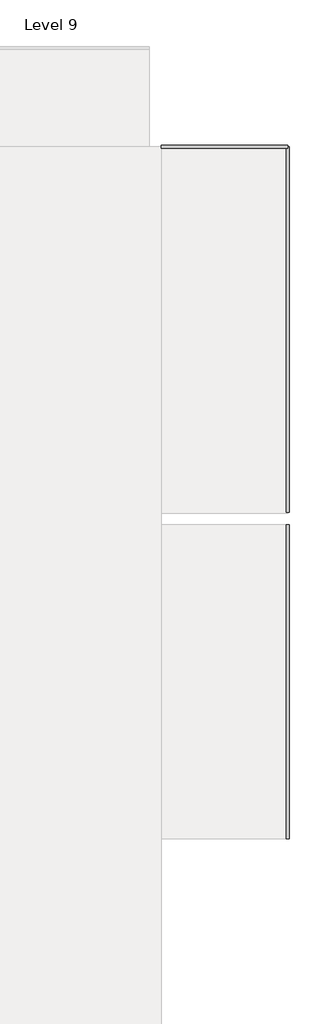
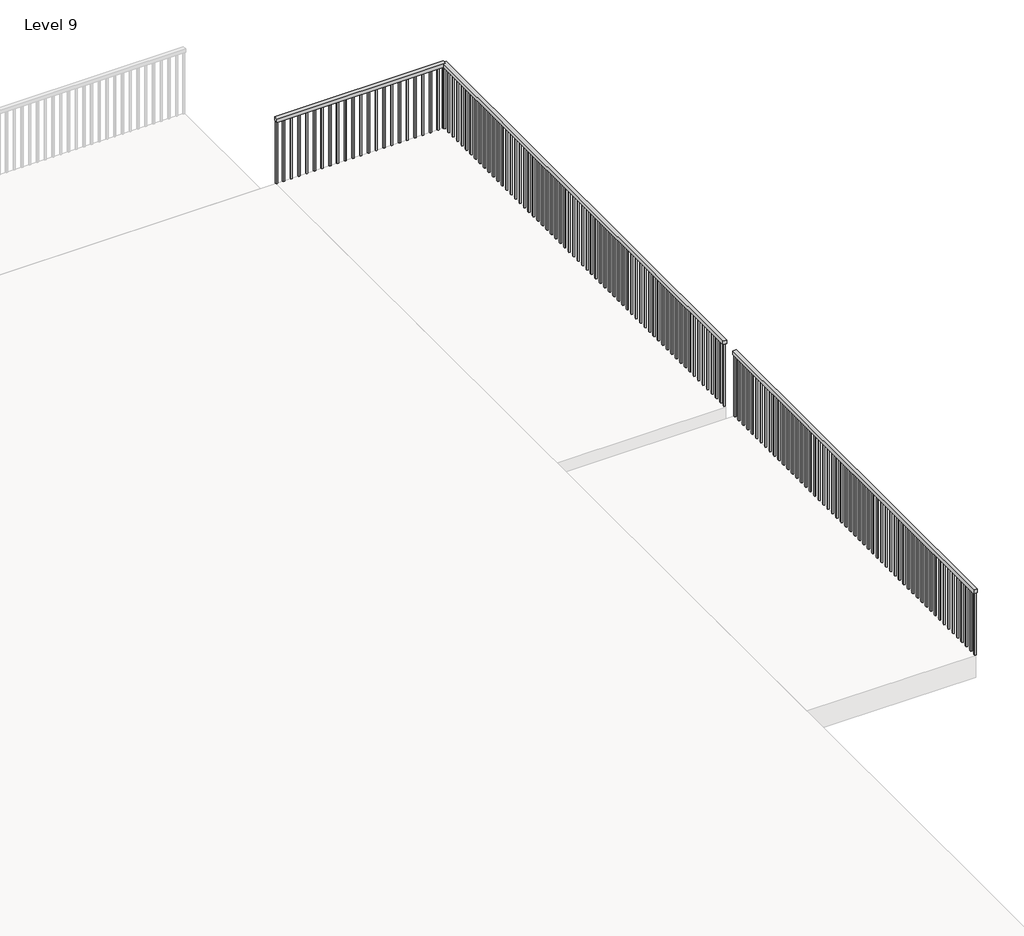
# One storey, part 4 of 5: 3 railings.
"""IFC4 building model written with IfcOpenShell, lengths in millimetres."""

from ifc_helpers import new_model, si_unit, frame, origin, place, context, project, spatial, polyline, outline, extrude, element, save

model = new_model("IFC4")

# Units and contexts
model_context = context("Model", 3, world=origin())
ifc_project = project(units=[si_unit("LENGTHUNIT", "METRE", prefix="MILLI")], contexts=[model_context])

# Site, building, storey
site = spatial("IfcSite", under=ifc_project)
building = spatial("IfcBuilding", under=site)
storey = spatial("IfcBuildingStorey", under=building, Name="Level 9", Elevation=9448.8)

# Railings
placement = place(None, origin())
element("IfcRailing", 1, ObjectType="Handrail - Rectangular", at=placement, inside=storey, context=model_context, shape_type="SweptSolid", body=[
    extrude(outline(polyline([(14106.5361222, 14743.2237525), (14106.5361222, 14794.0237525), (16321.4289933, 14794.0237525), (16321.4289933, 14743.2237525), (14106.5361222, 14743.2237525)])), frame((0.0, 0.0, 10312.4), z_axis=(0.0, 0.0, 1.0), x_axis=(1.0, 0.0, 0.0)), (0.0, 0.0, 1.0), 50.8),
    extrude(outline(polyline([(16230.6111222, 14759.0987525), (16230.6111222, 14778.1487525), (16249.6611222, 14778.1487525), (16249.6611222, 14759.0987525), (16230.6111222, 14759.0987525)])), frame((0.0, 0.0, 9448.8), z_axis=(0.0, 0.0, 1.0), x_axis=(1.0, 0.0, 0.0)), (0.0, 0.0, 1.0), 863.6),
    extrude(outline(polyline([(16129.0111222, 14759.0987525), (16129.0111222, 14778.1487525), (16148.0611222, 14778.1487525), (16148.0611222, 14759.0987525), (16129.0111222, 14759.0987525)])), frame((0.0, 0.0, 9448.8), z_axis=(0.0, 0.0, 1.0), x_axis=(1.0, 0.0, 0.0)), (0.0, 0.0, 1.0), 863.6),
    extrude(outline(polyline([(16027.4111222, 14759.0987525), (16027.4111222, 14778.1487525), (16046.4611222, 14778.1487525), (16046.4611222, 14759.0987525), (16027.4111222, 14759.0987525)])), frame((0.0, 0.0, 9448.8), z_axis=(0.0, 0.0, 1.0), x_axis=(1.0, 0.0, 0.0)), (0.0, 0.0, 1.0), 863.6),
    extrude(outline(polyline([(15925.8111222, 14759.0987525), (15925.8111222, 14778.1487525), (15944.8611222, 14778.1487525), (15944.8611222, 14759.0987525), (15925.8111222, 14759.0987525)])), frame((0.0, 0.0, 9448.8), z_axis=(0.0, 0.0, 1.0), x_axis=(1.0, 0.0, 0.0)), (0.0, 0.0, 1.0), 863.6),
    extrude(outline(polyline([(15824.2111222, 14759.0987525), (15824.2111222, 14778.1487525), (15843.2611222, 14778.1487525), (15843.2611222, 14759.0987525), (15824.2111222, 14759.0987525)])), frame((0.0, 0.0, 9448.8), z_axis=(0.0, 0.0, 1.0), x_axis=(1.0, 0.0, 0.0)), (0.0, 0.0, 1.0), 863.6),
    extrude(outline(polyline([(15722.6111222, 14759.0987525), (15722.6111222, 14778.1487525), (15741.6611222, 14778.1487525), (15741.6611222, 14759.0987525), (15722.6111222, 14759.0987525)])), frame((0.0, 0.0, 9448.8), z_axis=(0.0, 0.0, 1.0), x_axis=(1.0, 0.0, 0.0)), (0.0, 0.0, 1.0), 863.6),
    extrude(outline(polyline([(15621.0111222, 14759.0987525), (15621.0111222, 14778.1487525), (15640.0611222, 14778.1487525), (15640.0611222, 14759.0987525), (15621.0111222, 14759.0987525)])), frame((0.0, 0.0, 9448.8), z_axis=(0.0, 0.0, 1.0), x_axis=(1.0, 0.0, 0.0)), (0.0, 0.0, 1.0), 863.6),
    extrude(outline(polyline([(15519.4111222, 14759.0987525), (15519.4111222, 14778.1487525), (15538.4611222, 14778.1487525), (15538.4611222, 14759.0987525), (15519.4111222, 14759.0987525)])), frame((0.0, 0.0, 9448.8), z_axis=(0.0, 0.0, 1.0), x_axis=(1.0, 0.0, 0.0)), (0.0, 0.0, 1.0), 863.6),
    extrude(outline(polyline([(15417.8111222, 14759.0987525), (15417.8111222, 14778.1487525), (15436.8611222, 14778.1487525), (15436.8611222, 14759.0987525), (15417.8111222, 14759.0987525)])), frame((0.0, 0.0, 9448.8), z_axis=(0.0, 0.0, 1.0), x_axis=(1.0, 0.0, 0.0)), (0.0, 0.0, 1.0), 863.6),
    extrude(outline(polyline([(15316.2111222, 14759.0987525), (15316.2111222, 14778.1487525), (15335.2611222, 14778.1487525), (15335.2611222, 14759.0987525), (15316.2111222, 14759.0987525)])), frame((0.0, 0.0, 9448.8), z_axis=(0.0, 0.0, 1.0), x_axis=(1.0, 0.0, 0.0)), (0.0, 0.0, 1.0), 863.6),
    extrude(outline(polyline([(15214.6111222, 14759.0987525), (15214.6111222, 14778.1487525), (15233.6611222, 14778.1487525), (15233.6611222, 14759.0987525), (15214.6111222, 14759.0987525)])), frame((0.0, 0.0, 9448.8), z_axis=(0.0, 0.0, 1.0), x_axis=(1.0, 0.0, 0.0)), (0.0, 0.0, 1.0), 863.6),
    extrude(outline(polyline([(15113.0111222, 14759.0987525), (15113.0111222, 14778.1487525), (15132.0611222, 14778.1487525), (15132.0611222, 14759.0987525), (15113.0111222, 14759.0987525)])), frame((0.0, 0.0, 9448.8), z_axis=(0.0, 0.0, 1.0), x_axis=(1.0, 0.0, 0.0)), (0.0, 0.0, 1.0), 863.6),
    extrude(outline(polyline([(15011.4111222, 14759.0987525), (15011.4111222, 14778.1487525), (15030.4611222, 14778.1487525), (15030.4611222, 14759.0987525), (15011.4111222, 14759.0987525)])), frame((0.0, 0.0, 9448.8), z_axis=(0.0, 0.0, 1.0), x_axis=(1.0, 0.0, 0.0)), (0.0, 0.0, 1.0), 863.6),
    extrude(outline(polyline([(14909.8111222, 14759.0987525), (14909.8111222, 14778.1487525), (14928.8611222, 14778.1487525), (14928.8611222, 14759.0987525), (14909.8111222, 14759.0987525)])), frame((0.0, 0.0, 9448.8), z_axis=(0.0, 0.0, 1.0), x_axis=(1.0, 0.0, 0.0)), (0.0, 0.0, 1.0), 863.6),
    extrude(outline(polyline([(14808.2111222, 14759.0987525), (14808.2111222, 14778.1487525), (14827.2611222, 14778.1487525), (14827.2611222, 14759.0987525), (14808.2111222, 14759.0987525)])), frame((0.0, 0.0, 9448.8), z_axis=(0.0, 0.0, 1.0), x_axis=(1.0, 0.0, 0.0)), (0.0, 0.0, 1.0), 863.6),
    extrude(outline(polyline([(14706.6111222, 14759.0987525), (14706.6111222, 14778.1487525), (14725.6611222, 14778.1487525), (14725.6611222, 14759.0987525), (14706.6111222, 14759.0987525)])), frame((0.0, 0.0, 9448.8), z_axis=(0.0, 0.0, 1.0), x_axis=(1.0, 0.0, 0.0)), (0.0, 0.0, 1.0), 863.6),
    extrude(outline(polyline([(14605.0111222, 14759.0987525), (14605.0111222, 14778.1487525), (14624.0611222, 14778.1487525), (14624.0611222, 14759.0987525), (14605.0111222, 14759.0987525)])), frame((0.0, 0.0, 9448.8), z_axis=(0.0, 0.0, 1.0), x_axis=(1.0, 0.0, 0.0)), (0.0, 0.0, 1.0), 863.6),
    extrude(outline(polyline([(14503.4111222, 14759.0987525), (14503.4111222, 14778.1487525), (14522.4611222, 14778.1487525), (14522.4611222, 14759.0987525), (14503.4111222, 14759.0987525)])), frame((0.0, 0.0, 9448.8), z_axis=(0.0, 0.0, 1.0), x_axis=(1.0, 0.0, 0.0)), (0.0, 0.0, 1.0), 863.6),
    extrude(outline(polyline([(14401.8111222, 14759.0987525), (14401.8111222, 14778.1487525), (14420.8611222, 14778.1487525), (14420.8611222, 14759.0987525), (14401.8111222, 14759.0987525)])), frame((0.0, 0.0, 9448.8), z_axis=(0.0, 0.0, 1.0), x_axis=(1.0, 0.0, 0.0)), (0.0, 0.0, 1.0), 863.6),
    extrude(outline(polyline([(14300.2111222, 14759.0987525), (14300.2111222, 14778.1487525), (14319.2611222, 14778.1487525), (14319.2611222, 14759.0987525), (14300.2111222, 14759.0987525)])), frame((0.0, 0.0, 9448.8), z_axis=(0.0, 0.0, 1.0), x_axis=(1.0, 0.0, 0.0)), (0.0, 0.0, 1.0), 863.6),
    extrude(outline(polyline([(14198.6111222, 14759.0987525), (14198.6111222, 14778.1487525), (14217.6611222, 14778.1487525), (14217.6611222, 14759.0987525), (14198.6111222, 14759.0987525)])), frame((0.0, 0.0, 9448.8), z_axis=(0.0, 0.0, 1.0), x_axis=(1.0, 0.0, 0.0)), (0.0, 0.0, 1.0), 863.6),
    extrude(outline(polyline([(16302.3789933, 14759.0987525), (16302.3789933, 14778.1487525), (16321.4289933, 14778.1487525), (16321.4289933, 14759.0987525), (16302.3789933, 14759.0987525)])), frame((0.0, 0.0, 9448.8), z_axis=(0.0, 0.0, 1.0), x_axis=(1.0, 0.0, 0.0)), (0.0, 0.0, 1.0), 863.6),
    extrude(outline(polyline([(14106.5361222, 14759.0987525), (14106.5361222, 14778.1487525), (14125.5861222, 14778.1487525), (14125.5861222, 14759.0987525), (14106.5361222, 14759.0987525)])), frame((0.0, 0.0, 9448.8), z_axis=(0.0, 0.0, 1.0), x_axis=(1.0, 0.0, 0.0)), (0.0, 0.0, 1.0), 863.6),
])
element("IfcRailing", 2, ObjectType="Handrail - Rectangular", at=placement, inside=storey, context=model_context, shape_type="SweptSolid", body=[
    extrude(outline(polyline([(16296.0289933, 14768.6237525), (16346.8289933, 14768.6237525), (16346.8289933, 8386.8737525), (16296.0289933, 8386.8737525), (16296.0289933, 14768.6237525)])), frame((0.0, 0.0, 10312.4), z_axis=(0.0, 0.0, 1.0), x_axis=(1.0, 0.0, 0.0)), (0.0, 0.0, 1.0), 50.8),
    extrude(outline(polyline([(16311.9039933, 8478.9487525), (16330.9539933, 8478.9487525), (16330.9539933, 8459.8987525), (16311.9039933, 8459.8987525), (16311.9039933, 8478.9487525)])), frame((0.0, 0.0, 9448.8), z_axis=(0.0, 0.0, 1.0), x_axis=(1.0, 0.0, 0.0)), (0.0, 0.0, 1.0), 863.6),
    extrude(outline(polyline([(16311.9039933, 8580.5487525), (16330.9539933, 8580.5487525), (16330.9539933, 8561.4987525), (16311.9039933, 8561.4987525), (16311.9039933, 8580.5487525)])), frame((0.0, 0.0, 9448.8), z_axis=(0.0, 0.0, 1.0), x_axis=(1.0, 0.0, 0.0)), (0.0, 0.0, 1.0), 863.6),
    extrude(outline(polyline([(16311.9039933, 8682.1487525), (16330.9539933, 8682.1487525), (16330.9539933, 8663.0987525), (16311.9039933, 8663.0987525), (16311.9039933, 8682.1487525)])), frame((0.0, 0.0, 9448.8), z_axis=(0.0, 0.0, 1.0), x_axis=(1.0, 0.0, 0.0)), (0.0, 0.0, 1.0), 863.6),
    extrude(outline(polyline([(16311.9039933, 8783.7487525), (16330.9539933, 8783.7487525), (16330.9539933, 8764.6987525), (16311.9039933, 8764.6987525), (16311.9039933, 8783.7487525)])), frame((0.0, 0.0, 9448.8), z_axis=(0.0, 0.0, 1.0), x_axis=(1.0, 0.0, 0.0)), (0.0, 0.0, 1.0), 863.6),
    extrude(outline(polyline([(16311.9039933, 8885.3487525), (16330.9539933, 8885.3487525), (16330.9539933, 8866.2987525), (16311.9039933, 8866.2987525), (16311.9039933, 8885.3487525)])), frame((0.0, 0.0, 9448.8), z_axis=(0.0, 0.0, 1.0), x_axis=(1.0, 0.0, 0.0)), (0.0, 0.0, 1.0), 863.6),
    extrude(outline(polyline([(16311.9039933, 8986.9487525), (16330.9539933, 8986.9487525), (16330.9539933, 8967.8987525), (16311.9039933, 8967.8987525), (16311.9039933, 8986.9487525)])), frame((0.0, 0.0, 9448.8), z_axis=(0.0, 0.0, 1.0), x_axis=(1.0, 0.0, 0.0)), (0.0, 0.0, 1.0), 863.6),
    extrude(outline(polyline([(16311.9039933, 9088.5487525), (16330.9539933, 9088.5487525), (16330.9539933, 9069.4987525), (16311.9039933, 9069.4987525), (16311.9039933, 9088.5487525)])), frame((0.0, 0.0, 9448.8), z_axis=(0.0, 0.0, 1.0), x_axis=(1.0, 0.0, 0.0)), (0.0, 0.0, 1.0), 863.6),
    extrude(outline(polyline([(16311.9039933, 9190.1487525), (16330.9539933, 9190.1487525), (16330.9539933, 9171.0987525), (16311.9039933, 9171.0987525), (16311.9039933, 9190.1487525)])), frame((0.0, 0.0, 9448.8), z_axis=(0.0, 0.0, 1.0), x_axis=(1.0, 0.0, 0.0)), (0.0, 0.0, 1.0), 863.6),
    extrude(outline(polyline([(16311.9039933, 9291.7487525), (16330.9539933, 9291.7487525), (16330.9539933, 9272.6987525), (16311.9039933, 9272.6987525), (16311.9039933, 9291.7487525)])), frame((0.0, 0.0, 9448.8), z_axis=(0.0, 0.0, 1.0), x_axis=(1.0, 0.0, 0.0)), (0.0, 0.0, 1.0), 863.6),
    extrude(outline(polyline([(16311.9039933, 9393.3487525), (16330.9539933, 9393.3487525), (16330.9539933, 9374.2987525), (16311.9039933, 9374.2987525), (16311.9039933, 9393.3487525)])), frame((0.0, 0.0, 9448.8), z_axis=(0.0, 0.0, 1.0), x_axis=(1.0, 0.0, 0.0)), (0.0, 0.0, 1.0), 863.6),
    extrude(outline(polyline([(16311.9039933, 9494.9487525), (16330.9539933, 9494.9487525), (16330.9539933, 9475.8987525), (16311.9039933, 9475.8987525), (16311.9039933, 9494.9487525)])), frame((0.0, 0.0, 9448.8), z_axis=(0.0, 0.0, 1.0), x_axis=(1.0, 0.0, 0.0)), (0.0, 0.0, 1.0), 863.6),
    extrude(outline(polyline([(16311.9039933, 9596.5487525), (16330.9539933, 9596.5487525), (16330.9539933, 9577.4987525), (16311.9039933, 9577.4987525), (16311.9039933, 9596.5487525)])), frame((0.0, 0.0, 9448.8), z_axis=(0.0, 0.0, 1.0), x_axis=(1.0, 0.0, 0.0)), (0.0, 0.0, 1.0), 863.6),
    extrude(outline(polyline([(16311.9039933, 9698.1487525), (16330.9539933, 9698.1487525), (16330.9539933, 9679.0987525), (16311.9039933, 9679.0987525), (16311.9039933, 9698.1487525)])), frame((0.0, 0.0, 9448.8), z_axis=(0.0, 0.0, 1.0), x_axis=(1.0, 0.0, 0.0)), (0.0, 0.0, 1.0), 863.6),
    extrude(outline(polyline([(16311.9039933, 9799.7487525), (16330.9539933, 9799.7487525), (16330.9539933, 9780.6987525), (16311.9039933, 9780.6987525), (16311.9039933, 9799.7487525)])), frame((0.0, 0.0, 9448.8), z_axis=(0.0, 0.0, 1.0), x_axis=(1.0, 0.0, 0.0)), (0.0, 0.0, 1.0), 863.6),
    extrude(outline(polyline([(16311.9039933, 9901.3487525), (16330.9539933, 9901.3487525), (16330.9539933, 9882.2987525), (16311.9039933, 9882.2987525), (16311.9039933, 9901.3487525)])), frame((0.0, 0.0, 9448.8), z_axis=(0.0, 0.0, 1.0), x_axis=(1.0, 0.0, 0.0)), (0.0, 0.0, 1.0), 863.6),
    extrude(outline(polyline([(16311.9039933, 10002.9487525), (16330.9539933, 10002.9487525), (16330.9539933, 9983.8987525), (16311.9039933, 9983.8987525), (16311.9039933, 10002.9487525)])), frame((0.0, 0.0, 9448.8), z_axis=(0.0, 0.0, 1.0), x_axis=(1.0, 0.0, 0.0)), (0.0, 0.0, 1.0), 863.6),
    extrude(outline(polyline([(16311.9039933, 10104.5487525), (16330.9539933, 10104.5487525), (16330.9539933, 10085.4987525), (16311.9039933, 10085.4987525), (16311.9039933, 10104.5487525)])), frame((0.0, 0.0, 9448.8), z_axis=(0.0, 0.0, 1.0), x_axis=(1.0, 0.0, 0.0)), (0.0, 0.0, 1.0), 863.6),
    extrude(outline(polyline([(16311.9039933, 10206.1487525), (16330.9539933, 10206.1487525), (16330.9539933, 10187.0987525), (16311.9039933, 10187.0987525), (16311.9039933, 10206.1487525)])), frame((0.0, 0.0, 9448.8), z_axis=(0.0, 0.0, 1.0), x_axis=(1.0, 0.0, 0.0)), (0.0, 0.0, 1.0), 863.6),
    extrude(outline(polyline([(16311.9039933, 10307.7487525), (16330.9539933, 10307.7487525), (16330.9539933, 10288.6987525), (16311.9039933, 10288.6987525), (16311.9039933, 10307.7487525)])), frame((0.0, 0.0, 9448.8), z_axis=(0.0, 0.0, 1.0), x_axis=(1.0, 0.0, 0.0)), (0.0, 0.0, 1.0), 863.6),
    extrude(outline(polyline([(16311.9039933, 10409.3487525), (16330.9539933, 10409.3487525), (16330.9539933, 10390.2987525), (16311.9039933, 10390.2987525), (16311.9039933, 10409.3487525)])), frame((0.0, 0.0, 9448.8), z_axis=(0.0, 0.0, 1.0), x_axis=(1.0, 0.0, 0.0)), (0.0, 0.0, 1.0), 863.6),
    extrude(outline(polyline([(16311.9039933, 10510.9487525), (16330.9539933, 10510.9487525), (16330.9539933, 10491.8987525), (16311.9039933, 10491.8987525), (16311.9039933, 10510.9487525)])), frame((0.0, 0.0, 9448.8), z_axis=(0.0, 0.0, 1.0), x_axis=(1.0, 0.0, 0.0)), (0.0, 0.0, 1.0), 863.6),
    extrude(outline(polyline([(16311.9039933, 10612.5487525), (16330.9539933, 10612.5487525), (16330.9539933, 10593.4987525), (16311.9039933, 10593.4987525), (16311.9039933, 10612.5487525)])), frame((0.0, 0.0, 9448.8), z_axis=(0.0, 0.0, 1.0), x_axis=(1.0, 0.0, 0.0)), (0.0, 0.0, 1.0), 863.6),
    extrude(outline(polyline([(16311.9039933, 10714.1487525), (16330.9539933, 10714.1487525), (16330.9539933, 10695.0987525), (16311.9039933, 10695.0987525), (16311.9039933, 10714.1487525)])), frame((0.0, 0.0, 9448.8), z_axis=(0.0, 0.0, 1.0), x_axis=(1.0, 0.0, 0.0)), (0.0, 0.0, 1.0), 863.6),
    extrude(outline(polyline([(16311.9039933, 10815.7487525), (16330.9539933, 10815.7487525), (16330.9539933, 10796.6987525), (16311.9039933, 10796.6987525), (16311.9039933, 10815.7487525)])), frame((0.0, 0.0, 9448.8), z_axis=(0.0, 0.0, 1.0), x_axis=(1.0, 0.0, 0.0)), (0.0, 0.0, 1.0), 863.6),
    extrude(outline(polyline([(16311.9039933, 10917.3487525), (16330.9539933, 10917.3487525), (16330.9539933, 10898.2987525), (16311.9039933, 10898.2987525), (16311.9039933, 10917.3487525)])), frame((0.0, 0.0, 9448.8), z_axis=(0.0, 0.0, 1.0), x_axis=(1.0, 0.0, 0.0)), (0.0, 0.0, 1.0), 863.6),
    extrude(outline(polyline([(16311.9039933, 11018.9487525), (16330.9539933, 11018.9487525), (16330.9539933, 10999.8987525), (16311.9039933, 10999.8987525), (16311.9039933, 11018.9487525)])), frame((0.0, 0.0, 9448.8), z_axis=(0.0, 0.0, 1.0), x_axis=(1.0, 0.0, 0.0)), (0.0, 0.0, 1.0), 863.6),
    extrude(outline(polyline([(16311.9039933, 11120.5487525), (16330.9539933, 11120.5487525), (16330.9539933, 11101.4987525), (16311.9039933, 11101.4987525), (16311.9039933, 11120.5487525)])), frame((0.0, 0.0, 9448.8), z_axis=(0.0, 0.0, 1.0), x_axis=(1.0, 0.0, 0.0)), (0.0, 0.0, 1.0), 863.6),
    extrude(outline(polyline([(16311.9039933, 11222.1487525), (16330.9539933, 11222.1487525), (16330.9539933, 11203.0987525), (16311.9039933, 11203.0987525), (16311.9039933, 11222.1487525)])), frame((0.0, 0.0, 9448.8), z_axis=(0.0, 0.0, 1.0), x_axis=(1.0, 0.0, 0.0)), (0.0, 0.0, 1.0), 863.6),
    extrude(outline(polyline([(16311.9039933, 11323.7487525), (16330.9539933, 11323.7487525), (16330.9539933, 11304.6987525), (16311.9039933, 11304.6987525), (16311.9039933, 11323.7487525)])), frame((0.0, 0.0, 9448.8), z_axis=(0.0, 0.0, 1.0), x_axis=(1.0, 0.0, 0.0)), (0.0, 0.0, 1.0), 863.6),
    extrude(outline(polyline([(16311.9039933, 11425.3487525), (16330.9539933, 11425.3487525), (16330.9539933, 11406.2987525), (16311.9039933, 11406.2987525), (16311.9039933, 11425.3487525)])), frame((0.0, 0.0, 9448.8), z_axis=(0.0, 0.0, 1.0), x_axis=(1.0, 0.0, 0.0)), (0.0, 0.0, 1.0), 863.6),
    extrude(outline(polyline([(16311.9039933, 11526.9487525), (16330.9539933, 11526.9487525), (16330.9539933, 11507.8987525), (16311.9039933, 11507.8987525), (16311.9039933, 11526.9487525)])), frame((0.0, 0.0, 9448.8), z_axis=(0.0, 0.0, 1.0), x_axis=(1.0, 0.0, 0.0)), (0.0, 0.0, 1.0), 863.6),
    extrude(outline(polyline([(16311.9039933, 11628.5487525), (16330.9539933, 11628.5487525), (16330.9539933, 11609.4987525), (16311.9039933, 11609.4987525), (16311.9039933, 11628.5487525)])), frame((0.0, 0.0, 9448.8), z_axis=(0.0, 0.0, 1.0), x_axis=(1.0, 0.0, 0.0)), (0.0, 0.0, 1.0), 863.6),
    extrude(outline(polyline([(16311.9039933, 11730.1487525), (16330.9539933, 11730.1487525), (16330.9539933, 11711.0987525), (16311.9039933, 11711.0987525), (16311.9039933, 11730.1487525)])), frame((0.0, 0.0, 9448.8), z_axis=(0.0, 0.0, 1.0), x_axis=(1.0, 0.0, 0.0)), (0.0, 0.0, 1.0), 863.6),
    extrude(outline(polyline([(16311.9039933, 11831.7487525), (16330.9539933, 11831.7487525), (16330.9539933, 11812.6987525), (16311.9039933, 11812.6987525), (16311.9039933, 11831.7487525)])), frame((0.0, 0.0, 9448.8), z_axis=(0.0, 0.0, 1.0), x_axis=(1.0, 0.0, 0.0)), (0.0, 0.0, 1.0), 863.6),
    extrude(outline(polyline([(16311.9039933, 11933.3487525), (16330.9539933, 11933.3487525), (16330.9539933, 11914.2987525), (16311.9039933, 11914.2987525), (16311.9039933, 11933.3487525)])), frame((0.0, 0.0, 9448.8), z_axis=(0.0, 0.0, 1.0), x_axis=(1.0, 0.0, 0.0)), (0.0, 0.0, 1.0), 863.6),
    extrude(outline(polyline([(16311.9039933, 12034.9487525), (16330.9539933, 12034.9487525), (16330.9539933, 12015.8987525), (16311.9039933, 12015.8987525), (16311.9039933, 12034.9487525)])), frame((0.0, 0.0, 9448.8), z_axis=(0.0, 0.0, 1.0), x_axis=(1.0, 0.0, 0.0)), (0.0, 0.0, 1.0), 863.6),
    extrude(outline(polyline([(16311.9039933, 12136.5487525), (16330.9539933, 12136.5487525), (16330.9539933, 12117.4987525), (16311.9039933, 12117.4987525), (16311.9039933, 12136.5487525)])), frame((0.0, 0.0, 9448.8), z_axis=(0.0, 0.0, 1.0), x_axis=(1.0, 0.0, 0.0)), (0.0, 0.0, 1.0), 863.6),
    extrude(outline(polyline([(16311.9039933, 12238.1487525), (16330.9539933, 12238.1487525), (16330.9539933, 12219.0987525), (16311.9039933, 12219.0987525), (16311.9039933, 12238.1487525)])), frame((0.0, 0.0, 9448.8), z_axis=(0.0, 0.0, 1.0), x_axis=(1.0, 0.0, 0.0)), (0.0, 0.0, 1.0), 863.6),
    extrude(outline(polyline([(16311.9039933, 12339.7487525), (16330.9539933, 12339.7487525), (16330.9539933, 12320.6987525), (16311.9039933, 12320.6987525), (16311.9039933, 12339.7487525)])), frame((0.0, 0.0, 9448.8), z_axis=(0.0, 0.0, 1.0), x_axis=(1.0, 0.0, 0.0)), (0.0, 0.0, 1.0), 863.6),
    extrude(outline(polyline([(16311.9039933, 12441.3487525), (16330.9539933, 12441.3487525), (16330.9539933, 12422.2987525), (16311.9039933, 12422.2987525), (16311.9039933, 12441.3487525)])), frame((0.0, 0.0, 9448.8), z_axis=(0.0, 0.0, 1.0), x_axis=(1.0, 0.0, 0.0)), (0.0, 0.0, 1.0), 863.6),
    extrude(outline(polyline([(16311.9039933, 12542.9487525), (16330.9539933, 12542.9487525), (16330.9539933, 12523.8987525), (16311.9039933, 12523.8987525), (16311.9039933, 12542.9487525)])), frame((0.0, 0.0, 9448.8), z_axis=(0.0, 0.0, 1.0), x_axis=(1.0, 0.0, 0.0)), (0.0, 0.0, 1.0), 863.6),
    extrude(outline(polyline([(16311.9039933, 12644.5487525), (16330.9539933, 12644.5487525), (16330.9539933, 12625.4987525), (16311.9039933, 12625.4987525), (16311.9039933, 12644.5487525)])), frame((0.0, 0.0, 9448.8), z_axis=(0.0, 0.0, 1.0), x_axis=(1.0, 0.0, 0.0)), (0.0, 0.0, 1.0), 863.6),
    extrude(outline(polyline([(16311.9039933, 12746.1487525), (16330.9539933, 12746.1487525), (16330.9539933, 12727.0987525), (16311.9039933, 12727.0987525), (16311.9039933, 12746.1487525)])), frame((0.0, 0.0, 9448.8), z_axis=(0.0, 0.0, 1.0), x_axis=(1.0, 0.0, 0.0)), (0.0, 0.0, 1.0), 863.6),
    extrude(outline(polyline([(16311.9039933, 12847.7487525), (16330.9539933, 12847.7487525), (16330.9539933, 12828.6987525), (16311.9039933, 12828.6987525), (16311.9039933, 12847.7487525)])), frame((0.0, 0.0, 9448.8), z_axis=(0.0, 0.0, 1.0), x_axis=(1.0, 0.0, 0.0)), (0.0, 0.0, 1.0), 863.6),
    extrude(outline(polyline([(16311.9039933, 12949.3487525), (16330.9539933, 12949.3487525), (16330.9539933, 12930.2987525), (16311.9039933, 12930.2987525), (16311.9039933, 12949.3487525)])), frame((0.0, 0.0, 9448.8), z_axis=(0.0, 0.0, 1.0), x_axis=(1.0, 0.0, 0.0)), (0.0, 0.0, 1.0), 863.6),
    extrude(outline(polyline([(16311.9039933, 13050.9487525), (16330.9539933, 13050.9487525), (16330.9539933, 13031.8987525), (16311.9039933, 13031.8987525), (16311.9039933, 13050.9487525)])), frame((0.0, 0.0, 9448.8), z_axis=(0.0, 0.0, 1.0), x_axis=(1.0, 0.0, 0.0)), (0.0, 0.0, 1.0), 863.6),
    extrude(outline(polyline([(16311.9039933, 13152.5487525), (16330.9539933, 13152.5487525), (16330.9539933, 13133.4987525), (16311.9039933, 13133.4987525), (16311.9039933, 13152.5487525)])), frame((0.0, 0.0, 9448.8), z_axis=(0.0, 0.0, 1.0), x_axis=(1.0, 0.0, 0.0)), (0.0, 0.0, 1.0), 863.6),
    extrude(outline(polyline([(16311.9039933, 13254.1487525), (16330.9539933, 13254.1487525), (16330.9539933, 13235.0987525), (16311.9039933, 13235.0987525), (16311.9039933, 13254.1487525)])), frame((0.0, 0.0, 9448.8), z_axis=(0.0, 0.0, 1.0), x_axis=(1.0, 0.0, 0.0)), (0.0, 0.0, 1.0), 863.6),
    extrude(outline(polyline([(16311.9039933, 13355.7487525), (16330.9539933, 13355.7487525), (16330.9539933, 13336.6987525), (16311.9039933, 13336.6987525), (16311.9039933, 13355.7487525)])), frame((0.0, 0.0, 9448.8), z_axis=(0.0, 0.0, 1.0), x_axis=(1.0, 0.0, 0.0)), (0.0, 0.0, 1.0), 863.6),
    extrude(outline(polyline([(16311.9039933, 13457.3487525), (16330.9539933, 13457.3487525), (16330.9539933, 13438.2987525), (16311.9039933, 13438.2987525), (16311.9039933, 13457.3487525)])), frame((0.0, 0.0, 9448.8), z_axis=(0.0, 0.0, 1.0), x_axis=(1.0, 0.0, 0.0)), (0.0, 0.0, 1.0), 863.6),
    extrude(outline(polyline([(16311.9039933, 13558.9487525), (16330.9539933, 13558.9487525), (16330.9539933, 13539.8987525), (16311.9039933, 13539.8987525), (16311.9039933, 13558.9487525)])), frame((0.0, 0.0, 9448.8), z_axis=(0.0, 0.0, 1.0), x_axis=(1.0, 0.0, 0.0)), (0.0, 0.0, 1.0), 863.6),
    extrude(outline(polyline([(16311.9039933, 13660.5487525), (16330.9539933, 13660.5487525), (16330.9539933, 13641.4987525), (16311.9039933, 13641.4987525), (16311.9039933, 13660.5487525)])), frame((0.0, 0.0, 9448.8), z_axis=(0.0, 0.0, 1.0), x_axis=(1.0, 0.0, 0.0)), (0.0, 0.0, 1.0), 863.6),
    extrude(outline(polyline([(16311.9039933, 13762.1487525), (16330.9539933, 13762.1487525), (16330.9539933, 13743.0987525), (16311.9039933, 13743.0987525), (16311.9039933, 13762.1487525)])), frame((0.0, 0.0, 9448.8), z_axis=(0.0, 0.0, 1.0), x_axis=(1.0, 0.0, 0.0)), (0.0, 0.0, 1.0), 863.6),
    extrude(outline(polyline([(16311.9039933, 13863.7487525), (16330.9539933, 13863.7487525), (16330.9539933, 13844.6987525), (16311.9039933, 13844.6987525), (16311.9039933, 13863.7487525)])), frame((0.0, 0.0, 9448.8), z_axis=(0.0, 0.0, 1.0), x_axis=(1.0, 0.0, 0.0)), (0.0, 0.0, 1.0), 863.6),
    extrude(outline(polyline([(16311.9039933, 13965.3487525), (16330.9539933, 13965.3487525), (16330.9539933, 13946.2987525), (16311.9039933, 13946.2987525), (16311.9039933, 13965.3487525)])), frame((0.0, 0.0, 9448.8), z_axis=(0.0, 0.0, 1.0), x_axis=(1.0, 0.0, 0.0)), (0.0, 0.0, 1.0), 863.6),
    extrude(outline(polyline([(16311.9039933, 14066.9487525), (16330.9539933, 14066.9487525), (16330.9539933, 14047.8987525), (16311.9039933, 14047.8987525), (16311.9039933, 14066.9487525)])), frame((0.0, 0.0, 9448.8), z_axis=(0.0, 0.0, 1.0), x_axis=(1.0, 0.0, 0.0)), (0.0, 0.0, 1.0), 863.6),
    extrude(outline(polyline([(16311.9039933, 14168.5487525), (16330.9539933, 14168.5487525), (16330.9539933, 14149.4987525), (16311.9039933, 14149.4987525), (16311.9039933, 14168.5487525)])), frame((0.0, 0.0, 9448.8), z_axis=(0.0, 0.0, 1.0), x_axis=(1.0, 0.0, 0.0)), (0.0, 0.0, 1.0), 863.6),
    extrude(outline(polyline([(16311.9039933, 14270.1487525), (16330.9539933, 14270.1487525), (16330.9539933, 14251.0987525), (16311.9039933, 14251.0987525), (16311.9039933, 14270.1487525)])), frame((0.0, 0.0, 9448.8), z_axis=(0.0, 0.0, 1.0), x_axis=(1.0, 0.0, 0.0)), (0.0, 0.0, 1.0), 863.6),
    extrude(outline(polyline([(16311.9039933, 14371.7487525), (16330.9539933, 14371.7487525), (16330.9539933, 14352.6987525), (16311.9039933, 14352.6987525), (16311.9039933, 14371.7487525)])), frame((0.0, 0.0, 9448.8), z_axis=(0.0, 0.0, 1.0), x_axis=(1.0, 0.0, 0.0)), (0.0, 0.0, 1.0), 863.6),
    extrude(outline(polyline([(16311.9039933, 14473.3487525), (16330.9539933, 14473.3487525), (16330.9539933, 14454.2987525), (16311.9039933, 14454.2987525), (16311.9039933, 14473.3487525)])), frame((0.0, 0.0, 9448.8), z_axis=(0.0, 0.0, 1.0), x_axis=(1.0, 0.0, 0.0)), (0.0, 0.0, 1.0), 863.6),
    extrude(outline(polyline([(16311.9039933, 14574.9487525), (16330.9539933, 14574.9487525), (16330.9539933, 14555.8987525), (16311.9039933, 14555.8987525), (16311.9039933, 14574.9487525)])), frame((0.0, 0.0, 9448.8), z_axis=(0.0, 0.0, 1.0), x_axis=(1.0, 0.0, 0.0)), (0.0, 0.0, 1.0), 863.6),
    extrude(outline(polyline([(16311.9039933, 14676.5487525), (16330.9539933, 14676.5487525), (16330.9539933, 14657.4987525), (16311.9039933, 14657.4987525), (16311.9039933, 14676.5487525)])), frame((0.0, 0.0, 9448.8), z_axis=(0.0, 0.0, 1.0), x_axis=(1.0, 0.0, 0.0)), (0.0, 0.0, 1.0), 863.6),
    extrude(outline(polyline([(16311.9039933, 8405.9237525), (16330.9539933, 8405.9237525), (16330.9539933, 8386.8737525), (16311.9039933, 8386.8737525), (16311.9039933, 8405.9237525)])), frame((0.0, 0.0, 9448.8), z_axis=(0.0, 0.0, 1.0), x_axis=(1.0, 0.0, 0.0)), (0.0, 0.0, 1.0), 863.6),
    extrude(outline(polyline([(16311.9039933, 14768.6237525), (16330.9539933, 14768.6237525), (16330.9539933, 14749.5737525), (16311.9039933, 14749.5737525), (16311.9039933, 14768.6237525)])), frame((0.0, 0.0, 9448.8), z_axis=(0.0, 0.0, 1.0), x_axis=(1.0, 0.0, 0.0)), (0.0, 0.0, 1.0), 863.6),
])
element("IfcRailing", 3, ObjectType="Handrail - Rectangular", at=placement, inside=storey, context=model_context, shape_type="SweptSolid", body=[
    extrude(outline(polyline([(16296.0289933, 8164.6237525), (16346.8289933, 8164.6237525), (16346.8289933, 2678.2237525), (16296.0289933, 2678.2237525), (16296.0289933, 8164.6237525)])), frame((0.0, 0.0, 10312.4), z_axis=(0.0, 0.0, 1.0), x_axis=(1.0, 0.0, 0.0)), (0.0, 0.0, 1.0), 50.8),
    extrude(outline(polyline([(16311.9039933, 2789.3487525), (16330.9539933, 2789.3487525), (16330.9539933, 2770.2987525), (16311.9039933, 2770.2987525), (16311.9039933, 2789.3487525)])), frame((0.0, 0.0, 9448.8), z_axis=(0.0, 0.0, 1.0), x_axis=(1.0, 0.0, 0.0)), (0.0, 0.0, 1.0), 863.6),
    extrude(outline(polyline([(16311.9039933, 2890.9487525), (16330.9539933, 2890.9487525), (16330.9539933, 2871.8987525), (16311.9039933, 2871.8987525), (16311.9039933, 2890.9487525)])), frame((0.0, 0.0, 9448.8), z_axis=(0.0, 0.0, 1.0), x_axis=(1.0, 0.0, 0.0)), (0.0, 0.0, 1.0), 863.6),
    extrude(outline(polyline([(16311.9039933, 2992.5487525), (16330.9539933, 2992.5487525), (16330.9539933, 2973.4987525), (16311.9039933, 2973.4987525), (16311.9039933, 2992.5487525)])), frame((0.0, 0.0, 9448.8), z_axis=(0.0, 0.0, 1.0), x_axis=(1.0, 0.0, 0.0)), (0.0, 0.0, 1.0), 863.6),
    extrude(outline(polyline([(16311.9039933, 3094.1487525), (16330.9539933, 3094.1487525), (16330.9539933, 3075.0987525), (16311.9039933, 3075.0987525), (16311.9039933, 3094.1487525)])), frame((0.0, 0.0, 9448.8), z_axis=(0.0, 0.0, 1.0), x_axis=(1.0, 0.0, 0.0)), (0.0, 0.0, 1.0), 863.6),
    extrude(outline(polyline([(16311.9039933, 3195.7487525), (16330.9539933, 3195.7487525), (16330.9539933, 3176.6987525), (16311.9039933, 3176.6987525), (16311.9039933, 3195.7487525)])), frame((0.0, 0.0, 9448.8), z_axis=(0.0, 0.0, 1.0), x_axis=(1.0, 0.0, 0.0)), (0.0, 0.0, 1.0), 863.6),
    extrude(outline(polyline([(16311.9039933, 3297.3487525), (16330.9539933, 3297.3487525), (16330.9539933, 3278.2987525), (16311.9039933, 3278.2987525), (16311.9039933, 3297.3487525)])), frame((0.0, 0.0, 9448.8), z_axis=(0.0, 0.0, 1.0), x_axis=(1.0, 0.0, 0.0)), (0.0, 0.0, 1.0), 863.6),
    extrude(outline(polyline([(16311.9039933, 3398.9487525), (16330.9539933, 3398.9487525), (16330.9539933, 3379.8987525), (16311.9039933, 3379.8987525), (16311.9039933, 3398.9487525)])), frame((0.0, 0.0, 9448.8), z_axis=(0.0, 0.0, 1.0), x_axis=(1.0, 0.0, 0.0)), (0.0, 0.0, 1.0), 863.6),
    extrude(outline(polyline([(16311.9039933, 3500.5487525), (16330.9539933, 3500.5487525), (16330.9539933, 3481.4987525), (16311.9039933, 3481.4987525), (16311.9039933, 3500.5487525)])), frame((0.0, 0.0, 9448.8), z_axis=(0.0, 0.0, 1.0), x_axis=(1.0, 0.0, 0.0)), (0.0, 0.0, 1.0), 863.6),
    extrude(outline(polyline([(16311.9039933, 3602.1487525), (16330.9539933, 3602.1487525), (16330.9539933, 3583.0987525), (16311.9039933, 3583.0987525), (16311.9039933, 3602.1487525)])), frame((0.0, 0.0, 9448.8), z_axis=(0.0, 0.0, 1.0), x_axis=(1.0, 0.0, 0.0)), (0.0, 0.0, 1.0), 863.6),
    extrude(outline(polyline([(16311.9039933, 3703.7487525), (16330.9539933, 3703.7487525), (16330.9539933, 3684.6987525), (16311.9039933, 3684.6987525), (16311.9039933, 3703.7487525)])), frame((0.0, 0.0, 9448.8), z_axis=(0.0, 0.0, 1.0), x_axis=(1.0, 0.0, 0.0)), (0.0, 0.0, 1.0), 863.6),
    extrude(outline(polyline([(16311.9039933, 3805.3487525), (16330.9539933, 3805.3487525), (16330.9539933, 3786.2987525), (16311.9039933, 3786.2987525), (16311.9039933, 3805.3487525)])), frame((0.0, 0.0, 9448.8), z_axis=(0.0, 0.0, 1.0), x_axis=(1.0, 0.0, 0.0)), (0.0, 0.0, 1.0), 863.6),
    extrude(outline(polyline([(16311.9039933, 3906.9487525), (16330.9539933, 3906.9487525), (16330.9539933, 3887.8987525), (16311.9039933, 3887.8987525), (16311.9039933, 3906.9487525)])), frame((0.0, 0.0, 9448.8), z_axis=(0.0, 0.0, 1.0), x_axis=(1.0, 0.0, 0.0)), (0.0, 0.0, 1.0), 863.6),
    extrude(outline(polyline([(16311.9039933, 4008.5487525), (16330.9539933, 4008.5487525), (16330.9539933, 3989.4987525), (16311.9039933, 3989.4987525), (16311.9039933, 4008.5487525)])), frame((0.0, 0.0, 9448.8), z_axis=(0.0, 0.0, 1.0), x_axis=(1.0, 0.0, 0.0)), (0.0, 0.0, 1.0), 863.6),
    extrude(outline(polyline([(16311.9039933, 4110.1487525), (16330.9539933, 4110.1487525), (16330.9539933, 4091.0987525), (16311.9039933, 4091.0987525), (16311.9039933, 4110.1487525)])), frame((0.0, 0.0, 9448.8), z_axis=(0.0, 0.0, 1.0), x_axis=(1.0, 0.0, 0.0)), (0.0, 0.0, 1.0), 863.6),
    extrude(outline(polyline([(16311.9039933, 4211.7487525), (16330.9539933, 4211.7487525), (16330.9539933, 4192.6987525), (16311.9039933, 4192.6987525), (16311.9039933, 4211.7487525)])), frame((0.0, 0.0, 9448.8), z_axis=(0.0, 0.0, 1.0), x_axis=(1.0, 0.0, 0.0)), (0.0, 0.0, 1.0), 863.6),
    extrude(outline(polyline([(16311.9039933, 4313.3487525), (16330.9539933, 4313.3487525), (16330.9539933, 4294.2987525), (16311.9039933, 4294.2987525), (16311.9039933, 4313.3487525)])), frame((0.0, 0.0, 9448.8), z_axis=(0.0, 0.0, 1.0), x_axis=(1.0, 0.0, 0.0)), (0.0, 0.0, 1.0), 863.6),
    extrude(outline(polyline([(16311.9039933, 4414.9487525), (16330.9539933, 4414.9487525), (16330.9539933, 4395.8987525), (16311.9039933, 4395.8987525), (16311.9039933, 4414.9487525)])), frame((0.0, 0.0, 9448.8), z_axis=(0.0, 0.0, 1.0), x_axis=(1.0, 0.0, 0.0)), (0.0, 0.0, 1.0), 863.6),
    extrude(outline(polyline([(16311.9039933, 4516.5487525), (16330.9539933, 4516.5487525), (16330.9539933, 4497.4987525), (16311.9039933, 4497.4987525), (16311.9039933, 4516.5487525)])), frame((0.0, 0.0, 9448.8), z_axis=(0.0, 0.0, 1.0), x_axis=(1.0, 0.0, 0.0)), (0.0, 0.0, 1.0), 863.6),
    extrude(outline(polyline([(16311.9039933, 4618.1487525), (16330.9539933, 4618.1487525), (16330.9539933, 4599.0987525), (16311.9039933, 4599.0987525), (16311.9039933, 4618.1487525)])), frame((0.0, 0.0, 9448.8), z_axis=(0.0, 0.0, 1.0), x_axis=(1.0, 0.0, 0.0)), (0.0, 0.0, 1.0), 863.6),
    extrude(outline(polyline([(16311.9039933, 4719.7487525), (16330.9539933, 4719.7487525), (16330.9539933, 4700.6987525), (16311.9039933, 4700.6987525), (16311.9039933, 4719.7487525)])), frame((0.0, 0.0, 9448.8), z_axis=(0.0, 0.0, 1.0), x_axis=(1.0, 0.0, 0.0)), (0.0, 0.0, 1.0), 863.6),
    extrude(outline(polyline([(16311.9039933, 4821.3487525), (16330.9539933, 4821.3487525), (16330.9539933, 4802.2987525), (16311.9039933, 4802.2987525), (16311.9039933, 4821.3487525)])), frame((0.0, 0.0, 9448.8), z_axis=(0.0, 0.0, 1.0), x_axis=(1.0, 0.0, 0.0)), (0.0, 0.0, 1.0), 863.6),
    extrude(outline(polyline([(16311.9039933, 4922.9487525), (16330.9539933, 4922.9487525), (16330.9539933, 4903.8987525), (16311.9039933, 4903.8987525), (16311.9039933, 4922.9487525)])), frame((0.0, 0.0, 9448.8), z_axis=(0.0, 0.0, 1.0), x_axis=(1.0, 0.0, 0.0)), (0.0, 0.0, 1.0), 863.6),
    extrude(outline(polyline([(16311.9039933, 5024.5487525), (16330.9539933, 5024.5487525), (16330.9539933, 5005.4987525), (16311.9039933, 5005.4987525), (16311.9039933, 5024.5487525)])), frame((0.0, 0.0, 9448.8), z_axis=(0.0, 0.0, 1.0), x_axis=(1.0, 0.0, 0.0)), (0.0, 0.0, 1.0), 863.6),
    extrude(outline(polyline([(16311.9039933, 5126.1487525), (16330.9539933, 5126.1487525), (16330.9539933, 5107.0987525), (16311.9039933, 5107.0987525), (16311.9039933, 5126.1487525)])), frame((0.0, 0.0, 9448.8), z_axis=(0.0, 0.0, 1.0), x_axis=(1.0, 0.0, 0.0)), (0.0, 0.0, 1.0), 863.6),
    extrude(outline(polyline([(16311.9039933, 5227.7487525), (16330.9539933, 5227.7487525), (16330.9539933, 5208.6987525), (16311.9039933, 5208.6987525), (16311.9039933, 5227.7487525)])), frame((0.0, 0.0, 9448.8), z_axis=(0.0, 0.0, 1.0), x_axis=(1.0, 0.0, 0.0)), (0.0, 0.0, 1.0), 863.6),
    extrude(outline(polyline([(16311.9039933, 5329.3487525), (16330.9539933, 5329.3487525), (16330.9539933, 5310.2987525), (16311.9039933, 5310.2987525), (16311.9039933, 5329.3487525)])), frame((0.0, 0.0, 9448.8), z_axis=(0.0, 0.0, 1.0), x_axis=(1.0, 0.0, 0.0)), (0.0, 0.0, 1.0), 863.6),
    extrude(outline(polyline([(16311.9039933, 5430.9487525), (16330.9539933, 5430.9487525), (16330.9539933, 5411.8987525), (16311.9039933, 5411.8987525), (16311.9039933, 5430.9487525)])), frame((0.0, 0.0, 9448.8), z_axis=(0.0, 0.0, 1.0), x_axis=(1.0, 0.0, 0.0)), (0.0, 0.0, 1.0), 863.6),
    extrude(outline(polyline([(16311.9039933, 5532.5487525), (16330.9539933, 5532.5487525), (16330.9539933, 5513.4987525), (16311.9039933, 5513.4987525), (16311.9039933, 5532.5487525)])), frame((0.0, 0.0, 9448.8), z_axis=(0.0, 0.0, 1.0), x_axis=(1.0, 0.0, 0.0)), (0.0, 0.0, 1.0), 863.6),
    extrude(outline(polyline([(16311.9039933, 5634.1487525), (16330.9539933, 5634.1487525), (16330.9539933, 5615.0987525), (16311.9039933, 5615.0987525), (16311.9039933, 5634.1487525)])), frame((0.0, 0.0, 9448.8), z_axis=(0.0, 0.0, 1.0), x_axis=(1.0, 0.0, 0.0)), (0.0, 0.0, 1.0), 863.6),
    extrude(outline(polyline([(16311.9039933, 5735.7487525), (16330.9539933, 5735.7487525), (16330.9539933, 5716.6987525), (16311.9039933, 5716.6987525), (16311.9039933, 5735.7487525)])), frame((0.0, 0.0, 9448.8), z_axis=(0.0, 0.0, 1.0), x_axis=(1.0, 0.0, 0.0)), (0.0, 0.0, 1.0), 863.6),
    extrude(outline(polyline([(16311.9039933, 5837.3487525), (16330.9539933, 5837.3487525), (16330.9539933, 5818.2987525), (16311.9039933, 5818.2987525), (16311.9039933, 5837.3487525)])), frame((0.0, 0.0, 9448.8), z_axis=(0.0, 0.0, 1.0), x_axis=(1.0, 0.0, 0.0)), (0.0, 0.0, 1.0), 863.6),
    extrude(outline(polyline([(16311.9039933, 5938.9487525), (16330.9539933, 5938.9487525), (16330.9539933, 5919.8987525), (16311.9039933, 5919.8987525), (16311.9039933, 5938.9487525)])), frame((0.0, 0.0, 9448.8), z_axis=(0.0, 0.0, 1.0), x_axis=(1.0, 0.0, 0.0)), (0.0, 0.0, 1.0), 863.6),
    extrude(outline(polyline([(16311.9039933, 6040.5487525), (16330.9539933, 6040.5487525), (16330.9539933, 6021.4987525), (16311.9039933, 6021.4987525), (16311.9039933, 6040.5487525)])), frame((0.0, 0.0, 9448.8), z_axis=(0.0, 0.0, 1.0), x_axis=(1.0, 0.0, 0.0)), (0.0, 0.0, 1.0), 863.6),
    extrude(outline(polyline([(16311.9039933, 6142.1487525), (16330.9539933, 6142.1487525), (16330.9539933, 6123.0987525), (16311.9039933, 6123.0987525), (16311.9039933, 6142.1487525)])), frame((0.0, 0.0, 9448.8), z_axis=(0.0, 0.0, 1.0), x_axis=(1.0, 0.0, 0.0)), (0.0, 0.0, 1.0), 863.6),
    extrude(outline(polyline([(16311.9039933, 6243.7487525), (16330.9539933, 6243.7487525), (16330.9539933, 6224.6987525), (16311.9039933, 6224.6987525), (16311.9039933, 6243.7487525)])), frame((0.0, 0.0, 9448.8), z_axis=(0.0, 0.0, 1.0), x_axis=(1.0, 0.0, 0.0)), (0.0, 0.0, 1.0), 863.6),
    extrude(outline(polyline([(16311.9039933, 6345.3487525), (16330.9539933, 6345.3487525), (16330.9539933, 6326.2987525), (16311.9039933, 6326.2987525), (16311.9039933, 6345.3487525)])), frame((0.0, 0.0, 9448.8), z_axis=(0.0, 0.0, 1.0), x_axis=(1.0, 0.0, 0.0)), (0.0, 0.0, 1.0), 863.6),
    extrude(outline(polyline([(16311.9039933, 6446.9487525), (16330.9539933, 6446.9487525), (16330.9539933, 6427.8987525), (16311.9039933, 6427.8987525), (16311.9039933, 6446.9487525)])), frame((0.0, 0.0, 9448.8), z_axis=(0.0, 0.0, 1.0), x_axis=(1.0, 0.0, 0.0)), (0.0, 0.0, 1.0), 863.6),
    extrude(outline(polyline([(16311.9039933, 6548.5487525), (16330.9539933, 6548.5487525), (16330.9539933, 6529.4987525), (16311.9039933, 6529.4987525), (16311.9039933, 6548.5487525)])), frame((0.0, 0.0, 9448.8), z_axis=(0.0, 0.0, 1.0), x_axis=(1.0, 0.0, 0.0)), (0.0, 0.0, 1.0), 863.6),
    extrude(outline(polyline([(16311.9039933, 6650.1487525), (16330.9539933, 6650.1487525), (16330.9539933, 6631.0987525), (16311.9039933, 6631.0987525), (16311.9039933, 6650.1487525)])), frame((0.0, 0.0, 9448.8), z_axis=(0.0, 0.0, 1.0), x_axis=(1.0, 0.0, 0.0)), (0.0, 0.0, 1.0), 863.6),
    extrude(outline(polyline([(16311.9039933, 6751.7487525), (16330.9539933, 6751.7487525), (16330.9539933, 6732.6987525), (16311.9039933, 6732.6987525), (16311.9039933, 6751.7487525)])), frame((0.0, 0.0, 9448.8), z_axis=(0.0, 0.0, 1.0), x_axis=(1.0, 0.0, 0.0)), (0.0, 0.0, 1.0), 863.6),
    extrude(outline(polyline([(16311.9039933, 6853.3487525), (16330.9539933, 6853.3487525), (16330.9539933, 6834.2987525), (16311.9039933, 6834.2987525), (16311.9039933, 6853.3487525)])), frame((0.0, 0.0, 9448.8), z_axis=(0.0, 0.0, 1.0), x_axis=(1.0, 0.0, 0.0)), (0.0, 0.0, 1.0), 863.6),
    extrude(outline(polyline([(16311.9039933, 6954.9487525), (16330.9539933, 6954.9487525), (16330.9539933, 6935.8987525), (16311.9039933, 6935.8987525), (16311.9039933, 6954.9487525)])), frame((0.0, 0.0, 9448.8), z_axis=(0.0, 0.0, 1.0), x_axis=(1.0, 0.0, 0.0)), (0.0, 0.0, 1.0), 863.6),
    extrude(outline(polyline([(16311.9039933, 7056.5487525), (16330.9539933, 7056.5487525), (16330.9539933, 7037.4987525), (16311.9039933, 7037.4987525), (16311.9039933, 7056.5487525)])), frame((0.0, 0.0, 9448.8), z_axis=(0.0, 0.0, 1.0), x_axis=(1.0, 0.0, 0.0)), (0.0, 0.0, 1.0), 863.6),
    extrude(outline(polyline([(16311.9039933, 7158.1487525), (16330.9539933, 7158.1487525), (16330.9539933, 7139.0987525), (16311.9039933, 7139.0987525), (16311.9039933, 7158.1487525)])), frame((0.0, 0.0, 9448.8), z_axis=(0.0, 0.0, 1.0), x_axis=(1.0, 0.0, 0.0)), (0.0, 0.0, 1.0), 863.6),
    extrude(outline(polyline([(16311.9039933, 7259.7487525), (16330.9539933, 7259.7487525), (16330.9539933, 7240.6987525), (16311.9039933, 7240.6987525), (16311.9039933, 7259.7487525)])), frame((0.0, 0.0, 9448.8), z_axis=(0.0, 0.0, 1.0), x_axis=(1.0, 0.0, 0.0)), (0.0, 0.0, 1.0), 863.6),
    extrude(outline(polyline([(16311.9039933, 7361.3487525), (16330.9539933, 7361.3487525), (16330.9539933, 7342.2987525), (16311.9039933, 7342.2987525), (16311.9039933, 7361.3487525)])), frame((0.0, 0.0, 9448.8), z_axis=(0.0, 0.0, 1.0), x_axis=(1.0, 0.0, 0.0)), (0.0, 0.0, 1.0), 863.6),
    extrude(outline(polyline([(16311.9039933, 7462.9487525), (16330.9539933, 7462.9487525), (16330.9539933, 7443.8987525), (16311.9039933, 7443.8987525), (16311.9039933, 7462.9487525)])), frame((0.0, 0.0, 9448.8), z_axis=(0.0, 0.0, 1.0), x_axis=(1.0, 0.0, 0.0)), (0.0, 0.0, 1.0), 863.6),
    extrude(outline(polyline([(16311.9039933, 7564.5487525), (16330.9539933, 7564.5487525), (16330.9539933, 7545.4987525), (16311.9039933, 7545.4987525), (16311.9039933, 7564.5487525)])), frame((0.0, 0.0, 9448.8), z_axis=(0.0, 0.0, 1.0), x_axis=(1.0, 0.0, 0.0)), (0.0, 0.0, 1.0), 863.6),
    extrude(outline(polyline([(16311.9039933, 7666.1487525), (16330.9539933, 7666.1487525), (16330.9539933, 7647.0987525), (16311.9039933, 7647.0987525), (16311.9039933, 7666.1487525)])), frame((0.0, 0.0, 9448.8), z_axis=(0.0, 0.0, 1.0), x_axis=(1.0, 0.0, 0.0)), (0.0, 0.0, 1.0), 863.6),
    extrude(outline(polyline([(16311.9039933, 7767.7487525), (16330.9539933, 7767.7487525), (16330.9539933, 7748.6987525), (16311.9039933, 7748.6987525), (16311.9039933, 7767.7487525)])), frame((0.0, 0.0, 9448.8), z_axis=(0.0, 0.0, 1.0), x_axis=(1.0, 0.0, 0.0)), (0.0, 0.0, 1.0), 863.6),
    extrude(outline(polyline([(16311.9039933, 7869.3487525), (16330.9539933, 7869.3487525), (16330.9539933, 7850.2987525), (16311.9039933, 7850.2987525), (16311.9039933, 7869.3487525)])), frame((0.0, 0.0, 9448.8), z_axis=(0.0, 0.0, 1.0), x_axis=(1.0, 0.0, 0.0)), (0.0, 0.0, 1.0), 863.6),
    extrude(outline(polyline([(16311.9039933, 7970.9487525), (16330.9539933, 7970.9487525), (16330.9539933, 7951.8987525), (16311.9039933, 7951.8987525), (16311.9039933, 7970.9487525)])), frame((0.0, 0.0, 9448.8), z_axis=(0.0, 0.0, 1.0), x_axis=(1.0, 0.0, 0.0)), (0.0, 0.0, 1.0), 863.6),
    extrude(outline(polyline([(16311.9039933, 8072.5487525), (16330.9539933, 8072.5487525), (16330.9539933, 8053.4987525), (16311.9039933, 8053.4987525), (16311.9039933, 8072.5487525)])), frame((0.0, 0.0, 9448.8), z_axis=(0.0, 0.0, 1.0), x_axis=(1.0, 0.0, 0.0)), (0.0, 0.0, 1.0), 863.6),
    extrude(outline(polyline([(16311.9039933, 2697.2737525), (16330.9539933, 2697.2737525), (16330.9539933, 2678.2237525), (16311.9039933, 2678.2237525), (16311.9039933, 2697.2737525)])), frame((0.0, 0.0, 9448.8), z_axis=(0.0, 0.0, 1.0), x_axis=(1.0, 0.0, 0.0)), (0.0, 0.0, 1.0), 863.6),
    extrude(outline(polyline([(16311.9039933, 8164.6237525), (16330.9539933, 8164.6237525), (16330.9539933, 8145.5737525), (16311.9039933, 8145.5737525), (16311.9039933, 8164.6237525)])), frame((0.0, 0.0, 9448.8), z_axis=(0.0, 0.0, 1.0), x_axis=(1.0, 0.0, 0.0)), (0.0, 0.0, 1.0), 863.6),
])

save(model, "model.ifc")

# Revit data of these elements
# Type "Handrail - Rectangular"
#   Assembly Code = "C2010400"
#   built-in parameter 1008612 = 0.0416667 (stored number, unit not read)
#   built-in parameter 1008611 = 0.0416667 (stored number, unit not read)
#   built-in parameter 1008609 = 0.333333 (stored number, unit not read)
#   built-in parameter 1008604 = 0.166667 (stored number, unit not read)
#   built-in parameter 1008603 = 0.166667 (stored number, unit not read)
#   Railing Height = 3' - 0"
#   built-in parameter 1008630 = 2
#   built-in parameter 1008610 = 2
#   built-in parameter 1008618 = Baluster - Square : 3/4"
# Elements 1, 2, 3 (IfcRailing, "Handrail - Rectangular")
#   Phase Created = New Construction
